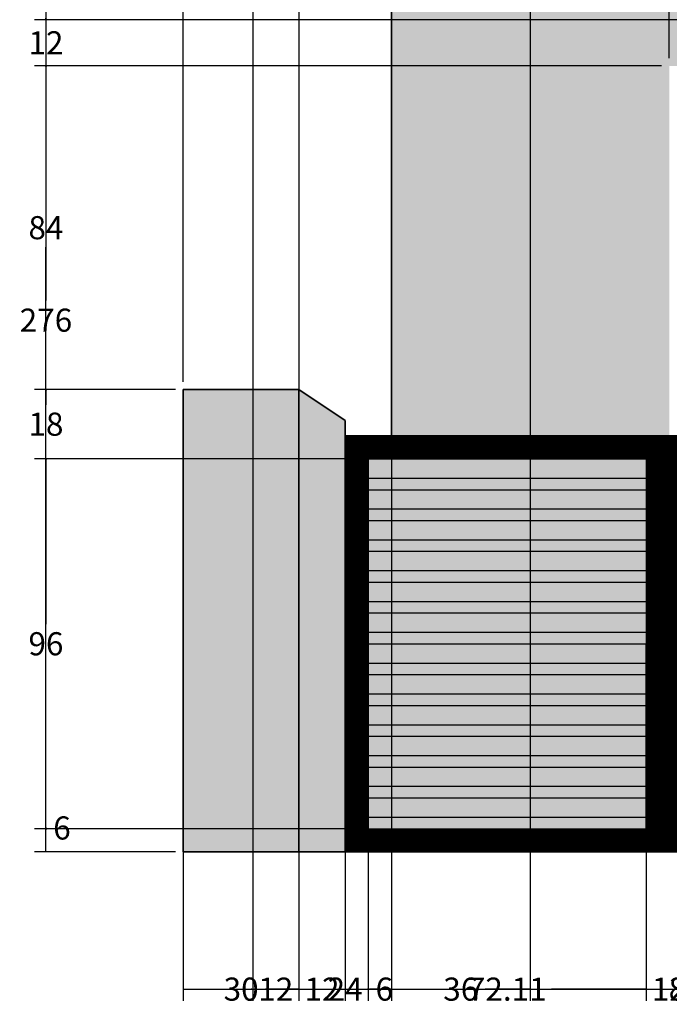
# Model space of a CAD drawing. Units: inches. Extents: x 860 to 1491, y 583 to 1370.
# Tile 1 of 8: x 866 to 1034, y 583 to 839. Entities that reach past the tile are written whole.
import ezdxf

# ---------------------------------------------------------------- set-up
doc = ezdxf.new("R2010")
doc.units = ezdxf.units.IN
doc.header["$MEASUREMENT"] = 0
doc.layers.get('0').update_dxf_attribs({"color": 250})
for name, color, linetype, lineweight in [('A-ANNO-DIMS', 2, 'Continuous', 18), ('A-ELEV', 7, 'Continuous', 35), ('A-ELEV-PATT', 9, 'Continuous', 13), ('A-SITE-GATE', 3, 'Continuous', 25), ('A-SITE-PATT', 8, 'Continuous', 13), ('A-SITE-WALL', 7, 'Continuous', 35)]:
    doc.layers.add(name, color=color, linetype=linetype, lineweight=lineweight)
doc.styles.get("Standard").update_dxf_attribs({"font": 'arial.ttf'})
doc.dimstyles.get("Standard").update_dxf_attribs({"dimtxt": 6, "dimasz": 0.18, "dimexe": 3, "dimexo": 2, "dimgap": 2, "dimtad": 0, "dimtih": 1, "dimtoh": 1, "dimdec": 0, "dimzin": 0, "dimdsep": 46, "dimlunit": 3, "dimtxsty": 'Standard', "dimblk2": 'CLOSEDBLANK', "dimsah": 1, "dimcen": 2, "dimadec": 0, "dimazin": 0, "dimtfac": 1, "dimtdec": 0, "dimtofl": 0, "dimtmove": 0, "dimatfit": 3, "dimfxl": 1, "dimtolj": 1, "dimtzin": 0, "dimarcsym": 0})

# ---------------------------------------------------------------- blocks, each defined once
blk = doc.blocks.new('_ClosedBlank')
at = {"color": 0, "linetype": 'ByBlock', "lineweight": -2}
for p, q in [((-1, 0.17), (0, 0)), ((-1, 0.17), (-1, -0.17)), ((0, 0), (-1, -0.17))]:
    blk.add_line(p, q, dxfattribs=at)
blk = doc.blocks.new('*D2')
at = {"layer": 'A-ANNO-DIMS', "color": 0, "lineweight": -2, "transparency": 16777216}
for p, q in [((1442.44, 1328.76), (1442.44, 584.11)), ((908.34, 740.76), (908.34, 584.11)), ((908.52, 587.11), (1163.85, 587.11)), ((1442.26, 587.11), (1186.93, 587.11))]:
    blk.add_line(p, q, dxfattribs=at)
at = {"layer": 'A-ANNO-DIMS', "color": 0, "transparency": 16777216}
blk.add_solid([(908.52, 587.14), (908.52, 587.08), (908.34, 587.11)], dxfattribs=at)
at = {"layer": 'Defpoints', "color": 0, "transparency": 16777216}
for p in [(1442.44, 1330.76), (908.34, 742.76), (1442.44, 587.11)]:
    blk.add_point(p, dxfattribs=at)
at = {"layer": 'A-ANNO-DIMS', "color": 0, "lineweight": -2, "transparency": 16777216, "xscale": 0.18, "yscale": 0.18, "zscale": 0.18}
blk.add_blockref('_ClosedBlank', (1442.44, 587.11), dxfattribs=at)
at = {"layer": 'A-ANNO-DIMS', "color": 0, "transparency": 16777216, "insert": (1175.39, 587.11), "char_height": 6, "attachment_point": 5}
blk.add_mtext('\\A1;534.1', dxfattribs=at)
blk = doc.blocks.new('*D4')
at = {"layer": 'A-ANNO-DIMS', "color": 0, "lineweight": -2, "transparency": 16777216}
for p, q in [((960.34, 898.76), (869.69, 898.76)), ((872.69, 898.58), (872.69, 765.82)), ((872.69, 622.94), (872.69, 755.69)), ((906.34, 622.76), (869.69, 622.76))]:
    blk.add_line(p, q, dxfattribs=at)
at = {"layer": 'A-ANNO-DIMS', "color": 0, "transparency": 16777216}
blk.add_solid([(872.66, 622.94), (872.72, 622.94), (872.69, 622.76)], dxfattribs=at)
at = {"layer": 'Defpoints', "color": 0, "transparency": 16777216}
for p in [(872.69, 898.76), (962.34, 898.76), (908.34, 622.76)]:
    blk.add_point(p, dxfattribs=at)
at = {"layer": 'A-ANNO-DIMS', "color": 0, "lineweight": -2, "transparency": 16777216, "xscale": 0.18, "yscale": 0.18, "zscale": 0.18, "rotation": 90}
blk.add_blockref('_ClosedBlank', (872.69, 898.76), dxfattribs=at)
at = {"layer": 'A-ANNO-DIMS', "color": 0, "transparency": 16777216, "insert": (872.69, 760.76), "char_height": 6, "attachment_point": 5}
blk.add_mtext('\\A1;276', dxfattribs=at)
blk = doc.blocks.new('*D6')
at = {"layer": 'A-ANNO-DIMS', "color": 0, "lineweight": -2, "transparency": 16777216}
for p, q in [((908.34, 740.76), (908.34, 584.11)), ((938.34, 740.76), (938.34, 584.11)), ((908.52, 587.11), (917.06, 587.11)), ((938.16, 587.11), (929.63, 587.11))]:
    blk.add_line(p, q, dxfattribs=at)
at = {"layer": 'A-ANNO-DIMS', "color": 0, "transparency": 16777216}
blk.add_solid([(908.52, 587.14), (908.52, 587.08), (908.34, 587.11)], dxfattribs=at)
at = {"layer": 'Defpoints', "color": 0, "transparency": 16777216}
for p in [(908.34, 742.76), (938.34, 742.76), (938.34, 587.11)]:
    blk.add_point(p, dxfattribs=at)
at = {"layer": 'A-ANNO-DIMS', "color": 0, "lineweight": -2, "transparency": 16777216, "xscale": 0.18, "yscale": 0.18, "zscale": 0.18}
blk.add_blockref('_ClosedBlank', (938.34, 587.11), dxfattribs=at)
at = {"layer": 'A-ANNO-DIMS', "color": 0, "transparency": 16777216, "insert": (923.34, 587.11), "char_height": 6, "attachment_point": 5}
blk.add_mtext('\\A1;30', dxfattribs=at)
blk = doc.blocks.new('*D7')
at = {"layer": 'A-ANNO-DIMS', "color": 0, "lineweight": -2, "transparency": 16777216}
for p, q in [((938.340309, 740.755507), (938.340309, 584.105507)), ((950.340309, 732.755507), (950.340309, 584.105507)), ((938.160309, 587.105507), (937.980309, 587.105507)), ((950.520309, 587.105507), (950.700309, 587.105507))]:
    blk.add_line(p, q, dxfattribs=at)
at = {"layer": 'A-ANNO-DIMS', "color": 0, "transparency": 16777216}
blk.add_solid([(938.160309, 587.135507), (938.160309, 587.075507), (938.340309, 587.105507)], dxfattribs=at)
at = {"layer": 'Defpoints', "color": 0, "transparency": 16777216}
for p in [(938.340309, 742.755507), (950.340309, 734.755507), (950.340309, 587.105507)]:
    blk.add_point(p, dxfattribs=at)
at = {"layer": 'A-ANNO-DIMS', "color": 0, "lineweight": -2, "transparency": 16777216, "xscale": 0.18, "yscale": 0.18, "zscale": 0.18, "rotation": 180}
blk.add_blockref('_ClosedBlank', (950.340309, 587.105507), dxfattribs=at)
at = {"layer": 'A-ANNO-DIMS', "color": 0, "transparency": 16777216, "insert": (944.340309, 587.105507), "char_height": 6, "attachment_point": 5}
blk.add_mtext('\\A1;12', dxfattribs=at)
blk = doc.blocks.new('*D8')
at = {"layer": 'A-ANNO-DIMS', "color": 0, "lineweight": -2, "transparency": 16777216}
for p, q in [((950.34, 732.76), (950.34, 584.11)), ((956.34, 722.76), (956.34, 584.11)), ((950.52, 587.11), (956.16, 587.11)), ((956.34, 587.11), (956.52, 587.11))]:
    blk.add_line(p, q, dxfattribs=at)
at = {"layer": 'A-ANNO-DIMS', "color": 0, "transparency": 16777216}
blk.add_solid([(950.52, 587.14), (950.52, 587.08), (950.34, 587.11)], dxfattribs=at)
at = {"layer": 'Defpoints', "color": 0, "transparency": 16777216}
for p in [(950.34, 734.76), (956.34, 724.76), (956.34, 587.11)]:
    blk.add_point(p, dxfattribs=at)
at = {"layer": 'A-ANNO-DIMS', "color": 0, "lineweight": -2, "transparency": 16777216, "xscale": 0.18, "yscale": 0.18, "zscale": 0.18}
blk.add_blockref('_ClosedBlank', (956.34, 587.11), dxfattribs=at)
at = {"layer": 'A-ANNO-DIMS', "color": 0, "transparency": 16777216, "insert": (960.5, 587.11), "char_height": 6, "attachment_point": 5}
blk.add_mtext('\\A1;6', dxfattribs=at)
blk = doc.blocks.new('*D9')
at = {"layer": 'A-ANNO-DIMS', "color": 0, "lineweight": -2, "transparency": 16777216}
for p, q in [((956.34, 722.76), (956.34, 584.11)), ((1028.45, 722.76), (1028.45, 584.11)), ((956.52, 587.11), (980.88, 587.11)), ((1028.27, 587.11), (1003.92, 587.11))]:
    blk.add_line(p, q, dxfattribs=at)
at = {"layer": 'A-ANNO-DIMS', "color": 0, "transparency": 16777216}
blk.add_solid([(956.52, 587.14), (956.52, 587.08), (956.34, 587.11)], dxfattribs=at)
at = {"layer": 'Defpoints', "color": 0, "transparency": 16777216}
for p in [(956.34, 724.76), (1028.45, 724.76), (1028.45, 587.11)]:
    blk.add_point(p, dxfattribs=at)
at = {"layer": 'A-ANNO-DIMS', "color": 0, "lineweight": -2, "transparency": 16777216, "xscale": 0.18, "yscale": 0.18, "zscale": 0.18}
blk.add_blockref('_ClosedBlank', (1028.45, 587.11), dxfattribs=at)
at = {"layer": 'A-ANNO-DIMS', "color": 0, "transparency": 16777216, "insert": (992.4, 587.11), "char_height": 6, "attachment_point": 5}
blk.add_mtext('\\A1;72.11', dxfattribs=at)
blk = doc.blocks.new('*D10')
at = {"layer": 'A-ANNO-DIMS', "color": 0, "lineweight": -2, "transparency": 16777216}
for p, q in [((1028.454444, 722.755507), (1028.454444, 584.105507)), ((1040.454446, 722.755507), (1040.454446, 584.105507)), ((1028.274444, 587.105507), (1028.094444, 587.105507)), ((1040.634446, 587.105507), (1040.814446, 587.105507))]:
    blk.add_line(p, q, dxfattribs=at)
at = {"layer": 'A-ANNO-DIMS', "color": 0, "transparency": 16777216}
blk.add_solid([(1028.274444, 587.135507), (1028.274444, 587.075507), (1028.454444, 587.105507)], dxfattribs=at)
at = {"layer": 'Defpoints', "color": 0, "transparency": 16777216}
for p in [(1028.454444, 724.755507), (1040.454446, 724.755507), (1040.454446, 587.105507)]:
    blk.add_point(p, dxfattribs=at)
at = {"layer": 'A-ANNO-DIMS', "color": 0, "lineweight": -2, "transparency": 16777216, "xscale": 0.18, "yscale": 0.18, "zscale": 0.18, "rotation": 180}
blk.add_blockref('_ClosedBlank', (1040.454446, 587.105507), dxfattribs=at)
at = {"layer": 'A-ANNO-DIMS', "color": 0, "transparency": 16777216, "insert": (1034.454445, 587.105507), "char_height": 6, "attachment_point": 5}
blk.add_mtext('\\A1;12', dxfattribs=at)
blk = doc.blocks.new('*D20')
at = {"layer": 'A-ANNO-DIMS', "color": 0, "lineweight": -2, "transparency": 16777216}
for p, q in [((908.34, 744.76), (908.34, 1369.41)), ((962.34, 732.76), (962.34, 1369.41)), ((908.52, 1366.41), (929.06, 1366.41)), ((962.16, 1366.41), (941.63, 1366.41))]:
    blk.add_line(p, q, dxfattribs=at)
at = {"layer": 'A-ANNO-DIMS', "color": 0, "transparency": 16777216}
blk.add_solid([(908.52, 1366.44), (908.52, 1366.38), (908.34, 1366.41)], dxfattribs=at)
at = {"layer": 'Defpoints', "color": 0, "transparency": 16777216}
for p in [(962.34, 1366.41), (908.34, 742.76), (962.34, 730.76)]:
    blk.add_point(p, dxfattribs=at)
at = {"layer": 'A-ANNO-DIMS', "color": 0, "lineweight": -2, "transparency": 16777216, "xscale": 0.18, "yscale": 0.18, "zscale": 0.18}
blk.add_blockref('_ClosedBlank', (962.34, 1366.41), dxfattribs=at)
at = {"layer": 'A-ANNO-DIMS', "color": 0, "transparency": 16777216, "insert": (935.34, 1366.41), "char_height": 6, "attachment_point": 5}
blk.add_mtext('\\A1;54', dxfattribs=at)
blk = doc.blocks.new('*D21')
at = {"layer": 'A-ANNO-DIMS', "color": 0, "lineweight": -2, "transparency": 16777216}
for p, q in [((962.34, 732.76), (962.34, 1369.41)), ((1034.46, 828.76), (1034.46, 1369.41)), ((962.52, 1366.41), (986.33, 1366.41)), ((1034.28, 1366.41), (1010.47, 1366.41))]:
    blk.add_line(p, q, dxfattribs=at)
at = {"layer": 'A-ANNO-DIMS', "color": 0, "transparency": 16777216}
blk.add_solid([(962.52, 1366.44), (962.52, 1366.38), (962.34, 1366.41)], dxfattribs=at)
at = {"layer": 'Defpoints', "color": 0, "transparency": 16777216}
for p in [(1034.46, 1366.41), (1034.46, 826.76), (962.34, 730.76)]:
    blk.add_point(p, dxfattribs=at)
at = {"layer": 'A-ANNO-DIMS', "color": 0, "lineweight": -2, "transparency": 16777216, "xscale": 0.18, "yscale": 0.18, "zscale": 0.18}
blk.add_blockref('_ClosedBlank', (1034.46, 1366.41), dxfattribs=at)
at = {"layer": 'A-ANNO-DIMS', "color": 0, "transparency": 16777216, "insert": (998.4, 1366.41), "char_height": 6, "attachment_point": 5}
blk.add_mtext('\\A1;72.12', dxfattribs=at)
blk = doc.blocks.new('*D22')
at = {"layer": 'A-ANNO-DIMS', "color": 0, "lineweight": -2, "transparency": 16777216}
for p, q in [((1034.46, 828.76), (1034.46, 1369.41)), ((1070.46, 828.76), (1070.46, 1369.41)), ((1034.64, 1366.41), (1046.17, 1366.41)), ((1070.28, 1366.41), (1058.75, 1366.41))]:
    blk.add_line(p, q, dxfattribs=at)
at = {"layer": 'A-ANNO-DIMS', "color": 0, "transparency": 16777216}
blk.add_solid([(1034.64, 1366.44), (1034.64, 1366.38), (1034.46, 1366.41)], dxfattribs=at)
at = {"layer": 'Defpoints', "color": 0, "transparency": 16777216}
for p in [(1070.46, 1366.41), (1034.46, 826.76), (1070.46, 826.76)]:
    blk.add_point(p, dxfattribs=at)
at = {"layer": 'A-ANNO-DIMS', "color": 0, "lineweight": -2, "transparency": 16777216, "xscale": 0.18, "yscale": 0.18, "zscale": 0.18}
blk.add_blockref('_ClosedBlank', (1070.46, 1366.41), dxfattribs=at)
at = {"layer": 'A-ANNO-DIMS', "color": 0, "transparency": 16777216, "insert": (1052.46, 1366.41), "char_height": 6, "attachment_point": 5}
blk.add_mtext('\\A1;36', dxfattribs=at)
blk = doc.blocks.new('*D31')
at = {"layer": 'A-ANNO-DIMS', "color": 0, "lineweight": -2, "transparency": 16777216}
for p, q in [((954.34, 628.76), (869.69, 628.76)), ((872.69, 628.76), (872.69, 628.94)), ((872.69, 628.94), (872.87, 628.94)), ((872.69, 622.94), (872.69, 628.58)), ((906.34, 622.76), (869.69, 622.76))]:
    blk.add_line(p, q, dxfattribs=at)
at = {"layer": 'A-ANNO-DIMS', "color": 0, "transparency": 16777216}
blk.add_solid([(872.66, 622.94), (872.72, 622.94), (872.69, 622.76)], dxfattribs=at)
at = {"layer": 'Defpoints', "color": 0, "transparency": 16777216}
for p in [(872.69, 628.76), (956.34, 628.76), (908.34, 622.76)]:
    blk.add_point(p, dxfattribs=at)
at = {"layer": 'A-ANNO-DIMS', "color": 0, "lineweight": -2, "transparency": 16777216, "xscale": 0.18, "yscale": 0.18, "zscale": 0.18, "rotation": 90}
blk.add_blockref('_ClosedBlank', (872.69, 628.76), dxfattribs=at)
at = {"layer": 'A-ANNO-DIMS', "color": 0, "transparency": 16777216, "insert": (876.85, 628.94), "char_height": 6, "attachment_point": 5}
blk.add_mtext('\\A1;6', dxfattribs=at)
blk = doc.blocks.new('*D32')
at = {"layer": 'A-ANNO-DIMS', "color": 0, "lineweight": -2, "transparency": 16777216}
for p, q in [((954.34, 724.76), (869.69, 724.76)), ((872.69, 724.58), (872.69, 681.82)), ((872.69, 628.94), (872.69, 671.69)), ((954.34, 628.76), (869.69, 628.76))]:
    blk.add_line(p, q, dxfattribs=at)
at = {"layer": 'A-ANNO-DIMS', "color": 0, "transparency": 16777216}
blk.add_solid([(872.66, 628.94), (872.72, 628.94), (872.69, 628.76)], dxfattribs=at)
at = {"layer": 'Defpoints', "color": 0, "transparency": 16777216}
for p in [(872.69, 724.76), (956.34, 724.76), (956.34, 628.76)]:
    blk.add_point(p, dxfattribs=at)
at = {"layer": 'A-ANNO-DIMS', "color": 0, "lineweight": -2, "transparency": 16777216, "xscale": 0.18, "yscale": 0.18, "zscale": 0.18, "rotation": 90}
blk.add_blockref('_ClosedBlank', (872.69, 724.76), dxfattribs=at)
at = {"layer": 'A-ANNO-DIMS', "color": 0, "transparency": 16777216, "insert": (872.69, 676.76), "char_height": 6, "attachment_point": 5}
blk.add_mtext('\\A1;96', dxfattribs=at)
blk = doc.blocks.new('*D33')
at = {"layer": 'A-ANNO-DIMS', "color": 0, "lineweight": -2, "transparency": 16777216}
for p, q in [((906.34, 742.76), (869.69, 742.76)), ((872.69, 742.58), (872.69, 738.82)), ((872.69, 724.94), (872.69, 728.69)), ((954.34, 724.76), (869.69, 724.76))]:
    blk.add_line(p, q, dxfattribs=at)
at = {"layer": 'A-ANNO-DIMS', "color": 0, "transparency": 16777216}
blk.add_solid([(872.66, 724.94), (872.72, 724.94), (872.69, 724.76)], dxfattribs=at)
at = {"layer": 'Defpoints', "color": 0, "transparency": 16777216}
for p in [(872.69, 742.76), (908.34, 742.76), (956.34, 724.76)]:
    blk.add_point(p, dxfattribs=at)
at = {"layer": 'A-ANNO-DIMS', "color": 0, "lineweight": -2, "transparency": 16777216, "xscale": 0.18, "yscale": 0.18, "zscale": 0.18, "rotation": 90}
blk.add_blockref('_ClosedBlank', (872.69, 742.76), dxfattribs=at)
at = {"layer": 'A-ANNO-DIMS', "color": 0, "transparency": 16777216, "insert": (872.69, 733.76), "char_height": 6, "attachment_point": 5}
blk.add_mtext('\\A1;18', dxfattribs=at)
blk = doc.blocks.new('*D34')
at = {"layer": 'A-ANNO-DIMS', "color": 0, "lineweight": -2, "transparency": 16777216}
for p, q in [((1032.46, 826.76), (869.69, 826.76)), ((872.69, 826.58), (872.69, 789.82)), ((872.69, 742.94), (872.69, 779.69)), ((906.34, 742.76), (869.69, 742.76))]:
    blk.add_line(p, q, dxfattribs=at)
at = {"layer": 'A-ANNO-DIMS', "color": 0, "transparency": 16777216}
blk.add_solid([(872.66, 742.94), (872.72, 742.94), (872.69, 742.76)], dxfattribs=at)
at = {"layer": 'Defpoints', "color": 0, "transparency": 16777216}
for p in [(872.69, 826.76), (1034.46, 826.76), (908.34, 742.76)]:
    blk.add_point(p, dxfattribs=at)
at = {"layer": 'A-ANNO-DIMS', "color": 0, "lineweight": -2, "transparency": 16777216, "xscale": 0.18, "yscale": 0.18, "zscale": 0.18, "rotation": 90}
blk.add_blockref('_ClosedBlank', (872.69, 826.76), dxfattribs=at)
at = {"layer": 'A-ANNO-DIMS', "color": 0, "transparency": 16777216, "insert": (872.69, 784.76), "char_height": 6, "attachment_point": 5}
blk.add_mtext('\\A1;84', dxfattribs=at)
blk = doc.blocks.new('*D35')
at = {"layer": 'A-ANNO-DIMS', "color": 0, "lineweight": -2, "transparency": 16777216}
for p, q in [((1116.440309, 838.755507), (869.690309, 838.755507)), ((872.690309, 838.935507), (872.690309, 839.115507)), ((1032.458453, 826.755507), (869.690309, 826.755507)), ((872.690309, 826.575507), (872.690309, 826.395507))]:
    blk.add_line(p, q, dxfattribs=at)
at = {"layer": 'A-ANNO-DIMS', "color": 0, "transparency": 16777216}
blk.add_solid([(872.660309, 826.575507), (872.720309, 826.575507), (872.690309, 826.755507)], dxfattribs=at)
at = {"layer": 'Defpoints', "color": 0, "transparency": 16777216}
for p in [(872.690309, 838.755507), (1118.440309, 838.755507), (1034.458453, 826.755507)]:
    blk.add_point(p, dxfattribs=at)
at = {"layer": 'A-ANNO-DIMS', "color": 0, "lineweight": -2, "transparency": 16777216, "xscale": 0.18, "yscale": 0.18, "zscale": 0.18, "rotation": 270}
blk.add_blockref('_ClosedBlank', (872.690309, 838.755507), dxfattribs=at)
at = {"layer": 'A-ANNO-DIMS', "color": 0, "transparency": 16777216, "insert": (872.690309, 832.755507), "char_height": 6, "attachment_point": 5}
blk.add_mtext('\\A1;12', dxfattribs=at)
blk = doc.blocks.new('*D62')
at = {"layer": 'A-ANNO-DIMS', "color": 0, "lineweight": -2, "transparency": 16777216}
for p, q in [((938.340309, 944.755507), (938.340309, 584.105507)), ((926.340309, 908.755507), (926.340309, 584.105507)), ((926.160309, 587.105507), (925.980309, 587.105507)), ((938.520309, 587.105507), (938.700309, 587.105507))]:
    blk.add_line(p, q, dxfattribs=at)
at = {"layer": 'A-ANNO-DIMS', "color": 0, "transparency": 16777216}
blk.add_solid([(926.160309, 587.135507), (926.160309, 587.075507), (926.340309, 587.105507)], dxfattribs=at)
at = {"layer": 'Defpoints', "color": 0, "transparency": 16777216}
for p in [(938.340309, 946.755507), (926.340309, 910.755507), (938.340309, 587.105507)]:
    blk.add_point(p, dxfattribs=at)
at = {"layer": 'A-ANNO-DIMS', "color": 0, "lineweight": -2, "transparency": 16777216, "xscale": 0.18, "yscale": 0.18, "zscale": 0.18, "rotation": 180}
blk.add_blockref('_ClosedBlank', (938.340309, 587.105507), dxfattribs=at)
at = {"layer": 'A-ANNO-DIMS', "color": 0, "transparency": 16777216, "insert": (932.340309, 587.105507), "char_height": 6, "attachment_point": 5}
blk.add_mtext('\\A1;12', dxfattribs=at)
blk = doc.blocks.new('*D63')
at = {"layer": 'A-ANNO-DIMS', "color": 0, "lineweight": -2, "transparency": 16777216}
for p, q in [((938.34, 944.76), (938.34, 584.11)), ((962.34, 881.35), (962.34, 584.11)), ((938.52, 587.11), (944, 587.11)), ((962.16, 587.11), (956.68, 587.11))]:
    blk.add_line(p, q, dxfattribs=at)
at = {"layer": 'A-ANNO-DIMS', "color": 0, "transparency": 16777216}
blk.add_solid([(938.52, 587.14), (938.52, 587.08), (938.34, 587.11)], dxfattribs=at)
at = {"layer": 'Defpoints', "color": 0, "transparency": 16777216}
for p in [(938.34, 946.76), (962.34, 883.35), (962.34, 587.11)]:
    blk.add_point(p, dxfattribs=at)
at = {"layer": 'A-ANNO-DIMS', "color": 0, "lineweight": -2, "transparency": 16777216, "xscale": 0.18, "yscale": 0.18, "zscale": 0.18}
blk.add_blockref('_ClosedBlank', (962.34, 587.11), dxfattribs=at)
at = {"layer": 'A-ANNO-DIMS', "color": 0, "transparency": 16777216, "insert": (950.34, 587.11), "char_height": 6, "attachment_point": 5}
blk.add_mtext('\\A1;24', dxfattribs=at)
blk = doc.blocks.new('*D64')
at = {"layer": 'A-ANNO-DIMS', "color": 0, "lineweight": -2, "transparency": 16777216}
for p, q in [((998.34, 956.76), (998.34, 584.11)), ((962.34, 881.35), (962.34, 584.11)), ((962.52, 587.11), (974.05, 587.11)), ((998.16, 587.11), (986.63, 587.11))]:
    blk.add_line(p, q, dxfattribs=at)
at = {"layer": 'A-ANNO-DIMS', "color": 0, "transparency": 16777216}
blk.add_solid([(962.52, 587.14), (962.52, 587.08), (962.34, 587.11)], dxfattribs=at)
at = {"layer": 'Defpoints', "color": 0, "transparency": 16777216}
for p in [(998.34, 958.76), (962.34, 883.35), (998.34, 587.11)]:
    blk.add_point(p, dxfattribs=at)
at = {"layer": 'A-ANNO-DIMS', "color": 0, "lineweight": -2, "transparency": 16777216, "xscale": 0.18, "yscale": 0.18, "zscale": 0.18}
blk.add_blockref('_ClosedBlank', (998.34, 587.11), dxfattribs=at)
at = {"layer": 'A-ANNO-DIMS', "color": 0, "transparency": 16777216, "insert": (980.34, 587.11), "char_height": 6, "attachment_point": 5}
blk.add_mtext('\\A1;36', dxfattribs=at)
blk = doc.blocks.new('*D65')
at = {"layer": 'A-ANNO-DIMS', "color": 0, "lineweight": -2, "transparency": 16777216}
for p, q in [((998.34, 956.76), (998.34, 584.11)), ((1079.34, 956.76), (1079.34, 584.11)), ((998.52, 587.11), (1033.12, 587.11)), ((1079.16, 587.11), (1044.56, 587.11))]:
    blk.add_line(p, q, dxfattribs=at)
at = {"layer": 'A-ANNO-DIMS', "color": 0, "transparency": 16777216}
blk.add_solid([(998.52, 587.14), (998.52, 587.08), (998.34, 587.11)], dxfattribs=at)
at = {"layer": 'Defpoints', "color": 0, "transparency": 16777216}
for p in [(998.34, 958.76), (1079.34, 958.76), (1079.34, 587.11)]:
    blk.add_point(p, dxfattribs=at)
at = {"layer": 'A-ANNO-DIMS', "color": 0, "lineweight": -2, "transparency": 16777216, "xscale": 0.18, "yscale": 0.18, "zscale": 0.18}
blk.add_blockref('_ClosedBlank', (1079.34, 587.11), dxfattribs=at)
at = {"layer": 'A-ANNO-DIMS', "color": 0, "transparency": 16777216, "insert": (1038.84, 587.11), "char_height": 6, "attachment_point": 5}
blk.add_mtext('\\A1;81', dxfattribs=at)

msp = doc.modelspace()

# ---------------------------------------------------------------- hatches: boundary and pattern name
at = {"layer": 'A-ELEV-PATT'}
h = msp.add_hatch(color=256, dxfattribs=at)
h.dxf.hatch_style = 1
h.paths.add_polyline_path([(1442.4403, 1330.7555), (1370.4403, 1330.7555), (1370.4403, 622.7555), (1442.4403, 622.7555)])
h.paths.add_polyline_path([(1358.4403, 1306.7555), (1190.4403, 1306.7555), (1190.4403, 1288.7555), (1358.4403, 1288.7555)])
h.paths.add_polyline_path([(1190.4403, 1234.7555), (962.3403, 1234.7555), (962.3403, 1198.7555), (1202.4403, 1198.7555), (1202.4403, 1216.7555), (1190.4403, 1216.7555)])
h.paths.add_polyline_path([(1202.4403, 1117.6207), (962.3403, 1117.6207), (962.3403, 982.7555), (986.3403, 982.7555), (986.3403, 1090.7555), (1178.3403, 1090.7555), (1178.3403, 982.7555), (1202.4403, 982.7555)])
h.paths.add_polyline_path([(1319.4403, 1184.7555), (1202.4403, 1184.7555), (1202.4403, 982.7555), (1211.4403, 982.7555), (1211.4403, 946.7555), (1220.4403, 946.7555), (1220.4403, 934.7555), (1319.4403, 934.7555)])
h.paths.add_polyline_path([(1271.4403, 1160.7555), (1307.4403, 1160.7555), (1307.4403, 944.7555), (1271.4403, 944.7555)], flags=16)
h.paths.add_polyline_path([(1275.4403, 1156.7555), (1303.4403, 1156.7555), (1303.4403, 948.7555), (1275.4403, 948.7555)], flags=0)
h.paths.add_polyline_path([(1202.4403, 898.7555), (962.3403, 898.7555), (962.3403, 730.7555), (1034.4585, 730.7555), (1034.4585, 826.7555), (1070.4585, 826.7555), (1070.4585, 730.7555), (1118.4403, 730.7555), (1118.4403, 838.7555), (1178.4403, 838.7555), (1178.4403, 730.7555), (1202.4403, 730.7555)])
h.paths.add_polyline_path([(1220.4403, 946.7555), (1211.4403, 946.7555), (938.3403, 946.7555), (926.3403, 946.7555), (926.3403, 910.7555), (962.3403, 910.7555), (1220.4403, 910.7555)])
h.paths.add_polyline_path([(950.3403, 730.7555), (950.3403, 734.7555), (938.3403, 742.7555), (938.3403, 730.7555), (938.3403, 622.7555), (950.3403, 622.7555)])
h = msp.add_hatch(color=256, dxfattribs=at)
h.dxf.hatch_style = 1
h.paths.add_polyline_path([(1370.4403, 730.7555), (1232.4403, 730.7555), (1232.4403, 622.7555), (1370.4403, 622.7555)])
h.paths.add_polyline_path([(1232.4403, 730.7555), (1232.4403, 742.7555), (1202.4403, 742.7555), (1202.4403, 622.7555), (1232.4403, 622.7555)])
h.paths.add_polyline_path([(1148.4403, 730.7555), (1148.4403, 742.7555), (1118.4403, 742.7555), (1118.4403, 718.7555), (1118.4403, 622.7555), (1148.4403, 622.7555)])
h.paths.add_polyline_path([(938.3403, 730.7555), (938.3403, 742.7555), (908.3403, 742.7555), (908.3403, 736.7555), (908.3403, 622.7555), (938.3403, 622.7555)])
h = msp.add_hatch(color=256, dxfattribs=at)
h.paths.add_polyline_path([(1040.4544, 724.7555), (1040.4511, 719.7555), (1112.4403, 719.7555), (1112.4403, 724.7555)])
h.paths.add_polyline_path([(1028.4511, 719.7555), (1028.4544, 724.7555), (956.3403, 724.7555), (956.3403, 719.7555)])
h.paths.add_polyline_path([(1028.4458, 711.7555), (1028.4491, 716.7555), (956.3403, 716.7555), (956.3403, 711.7555)])
h.paths.add_polyline_path([(1040.4491, 716.7555), (1040.4458, 711.7555), (1112.4403, 711.7555), (1112.4403, 716.7555)])
h.paths.add_polyline_path([(1040.4438, 708.7555), (1040.4404, 703.7555), (1112.4403, 703.7555), (1112.4403, 708.7555)])
h.paths.add_polyline_path([(1028.4351, 695.7555), (1028.4384, 700.7555), (956.3403, 700.7555), (956.3403, 695.7555)])
h.paths.add_polyline_path([(1040.4331, 692.7555), (1040.4297, 687.7555), (1112.4403, 687.7555), (1112.4403, 692.7555)])
h.paths.add_polyline_path([(1040.4224, 676.7555), (1040.419, 671.7555), (1112.4403, 671.7555), (1112.4403, 676.7555)])
h.paths.add_polyline_path([(1040.417, 668.7555), (1040.4137, 663.7555), (1112.4403, 663.7555), (1112.4403, 668.7555)])
h.paths.add_polyline_path([(1040.4063, 652.7555), (1040.403, 647.7555), (1112.4403, 647.7555), (1112.4403, 652.7555)])
h.paths.add_polyline_path([(1040.3957, 636.7555), (1040.3923, 631.7555), (1112.4403, 631.7555), (1112.4403, 636.7555)])
h = msp.add_hatch(color=256, dxfattribs=at)
h.paths.add_polyline_path([(1028.4511, 719.7555), (956.3403, 719.7555), (956.3403, 716.7555), (1028.4491, 716.7555)])
h.paths.add_polyline_path([(1028.4458, 711.7555), (956.3403, 711.7555), (956.3403, 708.7555), (1028.4438, 708.7555)])
h.paths.add_polyline_path([(1028.4404, 703.7555), (956.3403, 703.7555), (956.3403, 700.7555), (1028.4384, 700.7555)])
h.paths.add_polyline_path([(1028.4351, 695.7555), (956.3403, 695.7555), (956.3403, 692.7555), (1028.4331, 692.7555)])
h.paths.add_polyline_path([(1028.4297, 687.7555), (956.3403, 687.7555), (956.3403, 684.7555), (1028.4277, 684.7555)])
h.paths.add_polyline_path([(1028.4244, 679.7555), (956.3403, 679.7555), (956.3403, 676.7555), (1028.4224, 676.7555)])
h.paths.add_polyline_path([(1028.419, 671.7555), (956.3403, 671.7555), (956.3403, 668.7555), (1028.417, 668.7555)])
h.paths.add_polyline_path([(1028.4137, 663.7555), (956.3403, 663.7555), (956.3403, 660.7555), (1028.4117, 660.7555)])
h.paths.add_polyline_path([(1028.4083, 655.7555), (956.3403, 655.7555), (956.3403, 652.7555), (1028.4063, 652.7555)])
h.paths.add_polyline_path([(1028.403, 647.7555), (956.3403, 647.7555), (956.3403, 644.7555), (1028.401, 644.7555)])
h.paths.add_polyline_path([(1028.3977, 639.7555), (956.3403, 639.7555), (956.3403, 636.7555), (1028.3957, 636.7555)])
h.paths.add_polyline_path([(1028.3923, 631.7555), (956.3403, 631.7555), (956.3403, 628.7555), (1028.3903, 628.7074)])
h.paths.add_polyline_path([(1112.4403, 719.7555), (1040.4511, 719.7555), (1040.4491, 716.7555), (1112.4403, 716.7555)])
h.paths.add_polyline_path([(1112.4403, 711.7555), (1040.4458, 711.7555), (1040.4438, 708.7555), (1112.4403, 708.7555)])
h.paths.add_polyline_path([(1112.4403, 703.7555), (1040.4404, 703.7555), (1040.4384, 700.7555), (1112.4403, 700.7555)])
h.paths.add_polyline_path([(1112.4403, 695.7555), (1040.4351, 695.7555), (1040.4331, 692.7555), (1112.4403, 692.7555)])
h.paths.add_polyline_path([(1112.4403, 687.7555), (1040.4297, 687.7555), (1040.4277, 684.7555), (1112.4403, 684.7555)])
h.paths.add_polyline_path([(1112.4403, 679.7555), (1040.4244, 679.7555), (1040.4224, 676.7555), (1112.4403, 676.7555)])
h.paths.add_polyline_path([(1112.4403, 671.7555), (1040.419, 671.7555), (1040.417, 668.7555), (1112.4403, 668.7555)])
h.paths.add_polyline_path([(1112.4403, 663.7555), (1040.4137, 663.7555), (1040.4117, 660.7555), (1112.4403, 660.7555)])
h.paths.add_polyline_path([(1112.4403, 655.7555), (1040.4083, 655.7555), (1040.4063, 652.7555), (1112.4403, 652.7555)])
h.paths.add_polyline_path([(1112.4403, 647.7555), (1040.403, 647.7555), (1040.401, 644.7555), (1112.4403, 644.7555)])
h.paths.add_polyline_path([(1112.4403, 639.7555), (1040.3977, 639.7555), (1040.3957, 636.7555), (1112.4403, 636.7555)])
h.paths.add_polyline_path([(1112.4403, 631.7555), (1040.3923, 631.7555), (1040.3903, 628.7555), (1112.4403, 628.7555)])
h.paths.add_polyline_path([(1196.4403, 719.7555), (1154.4403, 719.7555), (1154.4403, 716.7555), (1196.4403, 716.7555)])
h.paths.add_polyline_path([(1196.4403, 711.7555), (1154.4403, 711.7555), (1154.4403, 708.7555), (1196.4403, 708.7555)])
h.paths.add_polyline_path([(1196.4403, 703.7555), (1154.4403, 703.7555), (1154.4403, 700.7555), (1196.4403, 700.7555)])
h.paths.add_polyline_path([(1196.4403, 695.7555), (1154.4403, 695.7555), (1154.4403, 692.7555), (1196.4403, 692.7555)])
h.paths.add_polyline_path([(1196.4403, 687.7555), (1154.4403, 687.7555), (1154.4403, 684.7555), (1196.4403, 684.7555)])
h.paths.add_polyline_path([(1196.4403, 679.7555), (1154.4403, 679.7555), (1154.4403, 676.7555), (1196.4403, 676.7555)])
h.paths.add_polyline_path([(1196.4403, 671.7555), (1154.4403, 671.7555), (1154.4403, 668.7555), (1196.4403, 668.7555)])
h.paths.add_polyline_path([(1196.4403, 663.7555), (1154.4403, 663.7555), (1154.4403, 660.7555), (1196.4403, 660.7555)])
h.paths.add_polyline_path([(1196.4403, 655.7555), (1154.4403, 655.7555), (1154.4403, 652.7555), (1196.4403, 652.7555)])
h.paths.add_polyline_path([(1196.4403, 647.7555), (1154.4403, 647.7555), (1154.4403, 644.7555), (1196.4403, 644.7555)])
h.paths.add_polyline_path([(1196.4403, 639.7555), (1154.4403, 639.7555), (1154.4403, 636.7555), (1196.4403, 636.7555)])
h.paths.add_polyline_path([(1196.4403, 631.7555), (1154.4403, 631.7555), (1154.4403, 628.7555), (1196.4403, 628.7555)])
h = msp.add_hatch(color=256, dxfattribs=at)
h.paths.add_polyline_path([(1028.4438, 708.7555), (956.3403, 708.7555), (956.3403, 703.7555), (1028.4404, 703.7555)])
h.paths.add_polyline_path([(1028.4331, 692.7555), (956.3403, 692.7555), (956.3403, 687.7555), (1028.4297, 687.7555)])
h.paths.add_polyline_path([(1028.4277, 684.7555), (956.3403, 684.7555), (956.3403, 679.7555), (1028.4244, 679.7555)])
h.paths.add_polyline_path([(1028.4224, 676.7555), (956.3403, 676.7555), (956.3403, 671.7555), (1028.419, 671.7555)])
h.paths.add_polyline_path([(1028.417, 668.7555), (956.3403, 668.7555), (956.3403, 663.7555), (1028.4137, 663.7555)])
h.paths.add_polyline_path([(1028.4117, 660.7555), (956.3403, 660.7555), (956.3403, 655.7555), (1028.4083, 655.7555)])
h.paths.add_polyline_path([(1028.4063, 652.7555), (956.3403, 652.7555), (956.3403, 647.7555), (1028.403, 647.7555)])
h.paths.add_polyline_path([(1028.401, 644.7555), (956.3403, 644.7555), (956.3403, 639.7555), (1028.3977, 639.7555)])
h.paths.add_polyline_path([(1028.3957, 636.7555), (956.3403, 636.7555), (956.3403, 631.7555), (1028.3923, 631.7555)])
h.paths.add_polyline_path([(1112.4403, 644.7555), (1040.401, 644.7555), (1040.3977, 639.7555), (1112.4403, 639.7555)])
h.paths.add_polyline_path([(1112.4403, 660.7555), (1040.4117, 660.7555), (1040.4083, 655.7555), (1112.4403, 655.7555)])
h.paths.add_polyline_path([(1112.4403, 684.7555), (1040.4277, 684.7555), (1040.4244, 679.7555), (1112.4403, 679.7555)])
h.paths.add_polyline_path([(1112.4403, 700.7555), (1040.4384, 700.7555), (1040.4351, 695.7555), (1112.4403, 695.7555)])
at = {"layer": 'A-SITE-PATT'}
h = msp.add_hatch(dxfattribs=at)
h.set_pattern_fill('GRAVEL', color=256, scale=30, style=0)
h.set_pattern_definition([(228.01279, (21.6, 30), (-240, -270), [4.0361, -399.57264]), (184.96974, (18.9, 27), (360, 30), [6.92604, -685.67774]), (132.51045, (12, 26.4), (300, -330), [4.88364, -483.481]), (267.27369, (0.3, 18.9), (30, 600), [6.30714, -624.40674]), (292.83365, (0, 12.6), (-150, 360), [6.18465, -612.2812]), (357.27369, (2.4, 6.9), (-600, 30), [6.30714, -624.40674]), (37.69424, (8.7, 6.6), (-390, -300), [8.34087, -825.74546]), (72.25533, (15.3, 11.7), (210, 660), [7.87464, -779.58964]), (121.42957, (17.7, 19.2), (-240, 390), [6.3285, -626.5222]), (175.23636, (14.4, 24.6), (330, -30), [7.22496, -354.0229]), (222.39744, (7.2, 25.2), (-360, -330), [9.34344, -925.00125]), (138.81407, (30, 18.6), (-210, 180), [3.18903, -315.71534]), (171.46923, (27.6, 20.7), (390, -60), [6.0671, -600.64534]), (225, (21.6, 21.6), (-3e-15, -30), [4.24263, -38.1838]), (203.1986, (19.5, 25.2), (150, 60), [2.28474, -226.18845]), (291.8014, (17.4, 24.3), (-30, 90), [3.2311, -158.32385]), (30.96376, (18.6, 21.3), (90, 60), [5.24787, -169.6807]), (161.56505, (23.1, 24), (60, -30), [3.79473, -91.0736]), (16.38954, (0, 24.3), (300, 90), [5.316, -526.28535]), (70.34618, (5.1, 25.8), (-120, -330), [4.45983, -441.52223]), (293.1986, (23.1, 30), (-60, 150), [4.56945, -223.90374]), (343.61046, (24.9, 25.8), (-300, 90), [5.316, -526.28535]), (339.44395, (0, 5.7), (-150, 60), [5.1264, -251.1937]), (294.77514, (4.8, 3.9), (-150, 330), [4.29534, -425.2393]), (66.8014, (23.4, 0), (60, 150), [4.56945, -223.90374]), (17.35402, (25.2, 4.2), (-390, -120), [5.02893, -497.8627]), (69.44395, (8.7, 0), (-60, -150), [2.5632, -253.7569]), (101.30993, (21.6, 0), (-30, 120), [1.5297, -151.4409]), (165.96376, (21.3, 1.5), (90, -30), [6.18465, -117.5085]), (186.00901, (15.3, 3), (300, 30), [5.7315, -567.4177]), (303.69007, (18.6, 18.6), (-30, 60), [4.32666, -103.8399]), (353.15723, (21, 15), (510, -60), [7.55382, -747.82688]), (60.9454, (28.5, 14.1), (-120, -210), [3.0887, -305.7802]), (90, (30, 16.8), (-30, 30), [1.8, -28.2]), (120.25644, (14.7, 3.9), (120, -210), [4.1677, -412.6056]), (48.01279, (12.6, 7.5), (240, 270), [8.07216, -395.53656]), (0, (18, 13.5), (30, 30), [7.8, -22.2]), (325.30485, (25.8, 13.5), (300, -210), [4.7434, -469.59823]), (254.0546, (29.7, 10.8), (-30, -120), [4.36806, -214.03524]), (207.64598, (28.5, 6.6), (-570, -300), [7.11195, -704.08423]), (175.42608, (22.2, 3.3), (-390, 30), [7.52397, -744.8722])])
h.paths.add_polyline_path([(1370.4403, 730.7555), (1232.4403, 730.7555), (1232.4403, 622.7555), (1370.4403, 622.7555)])
h.paths.add_polyline_path([(1232.4403, 730.7555), (1232.4403, 742.7555), (1202.4403, 742.7555), (1202.4403, 622.7555), (1232.4403, 622.7555)])
h.paths.add_polyline_path([(1148.4403, 730.7555), (1148.4403, 742.7555), (1118.4403, 742.7555), (1118.4403, 718.7555), (1118.4403, 622.7555), (1148.4403, 622.7555)])
h.paths.add_polyline_path([(938.3403, 730.7555), (938.3403, 742.7555), (908.3403, 742.7555), (908.3403, 736.7555), (908.3403, 622.7555), (938.3403, 622.7555)])
h = msp.add_hatch(dxfattribs=at)
h.set_pattern_fill('ANSI31', color=256, style=0)
h.paths.add_polyline_path([(1118.4403, 730.7555), (962.3403, 730.7555), (950.3403, 730.7555), (950.3403, 622.7555), (1118.4403, 622.7555)])
h.paths.add_polyline_path([(1028.4544, 724.7555), (1028.3903, 628.7074), (956.3403, 628.7555), (956.3403, 724.7555)], flags=16)
h.paths.add_polyline_path([(1040.4544, 724.7555), (1112.4403, 724.7555), (1112.4403, 628.7555), (1040.3903, 628.7555)], flags=16)
h.paths.add_polyline_path([(1202.4403, 730.7555), (1148.4403, 730.7555), (1148.4403, 622.7555), (1202.4403, 622.7555)])
h.paths.add_polyline_path([(1154.4403, 724.7555), (1196.4403, 724.7555), (1196.4403, 628.7555), (1154.4403, 628.7555)], flags=16)

# ---------------------------------------------------------------- linework, layer by layer
at = {"layer": 'A-ELEV'}
for p, q in [((962.3403, 730.7555), (962.3403, 898.7555)), ((938.3403, 742.7555), (908.3403, 742.7555)), ((908.3403, 742.7555), (908.3403, 736.7555)), ((938.3403, 730.7555), (938.3403, 742.7555)), ((950.3403, 734.7555), (938.3403, 742.7555)), ((908.3403, 622.7555), (908.3403, 736.7555)), ((950.3403, 730.7555), (950.3403, 734.7555))]:
    msp.add_line(p, q, dxfattribs=at)
at = {"layer": 'A-SITE-GATE'}
for p, q in [((956.3403, 724.7555), (956.3403, 628.7555)), ((956.3403, 724.7555), (1028.4544, 724.7555)), ((1028.4544, 724.7555), (1028.3903, 628.7595)), ((956.3403, 719.7555), (1028.4511, 719.7555)), ((956.3403, 716.7555), (1028.4491, 716.7555)), ((956.3403, 711.7555), (1028.4458, 711.7555)), ((956.3403, 708.7555), (1028.4438, 708.7555)), ((956.3403, 703.7555), (1028.4404, 703.7555)), ((956.3403, 700.7555), (1028.4384, 700.7555)), ((956.3403, 695.7555), (1028.4351, 695.7555)), ((956.3403, 692.7555), (1028.4331, 692.7555)), ((956.3403, 687.7555), (1028.4297, 687.7555)), ((956.3403, 684.7555), (1028.4277, 684.7555)), ((956.3403, 679.7555), (1028.4244, 679.7555)), ((956.3403, 676.7555), (1028.4224, 676.7555)), ((956.3403, 671.7555), (1028.419, 671.7555)), ((956.3403, 668.7555), (1028.417, 668.7555)), ((956.3403, 663.7555), (1028.4137, 663.7555)), ((956.3403, 660.7555), (1028.4117, 660.7555)), ((956.3403, 655.7555), (1028.4083, 655.7555)), ((956.3403, 652.7555), (1028.4063, 652.7555)), ((956.3403, 647.7555), (1028.403, 647.7555)), ((956.3403, 644.7555), (1028.401, 644.7555)), ((956.3403, 639.7555), (1028.3977, 639.7555)), ((956.3403, 636.7555), (1028.3957, 636.7555)), ((956.3403, 631.7555), (1028.3923, 631.7555)), ((956.3403, 628.7555), (1028.3903, 628.7074))]:
    msp.add_line(p, q, dxfattribs=at)
at = {"layer": 'A-SITE-WALL'}
for p, q in [((938.3403, 622.7555), (938.3403, 730.7555)), ((962.3403, 730.7555), (950.3403, 730.7555)), ((950.3403, 730.7555), (950.3403, 622.7555)), ((962.3403, 730.7555), (1118.4403, 730.7555)), ((1028.4585, 730.7595), (1028.4585, 730.7555)), ((908.3403, 622.7555), (1442.4403, 622.7555))]:
    msp.add_line(p, q, dxfattribs=at)

# ---------------------------------------------------------------- dimensions: what is measured, and where the dimension line sits
at = {"layer": 'A-ANNO-DIMS'}
for base, p1, p2, override, picture, middle in [((962.3403, 1366.4055), (908.3403, 742.7555), (962.3403, 730.7555), {"dimdec": 0, "dimlfac": 1, "dimrnd": 0, "dimzin": 0, "dimdsep": 46, "dimlunit": 2}, '*D20', (935.3403, 1366.4055)), ((1034.4585, 1366.4055), (962.3403, 730.7555), (1034.4585, 826.7555), {"dimdec": 2, "dimlfac": 1, "dimrnd": 0, "dimzin": 0, "dimdsep": 46, "dimlunit": 2}, '*D21', (998.3994, 1366.4055)), ((1070.4585, 1366.4055), (1034.4585, 826.7555), (1070.4585, 826.7555), {"dimdec": 0, "dimlfac": 1, "dimrnd": 0, "dimzin": 0, "dimdsep": 46, "dimlunit": 2}, '*D22', (1052.4585, 1366.4055)), ((1442.4403, 587.1055), (908.3403, 742.7555), (1442.4403, 1330.7555), {"dimdec": 1, "dimlfac": 1, "dimrnd": 0, "dimzin": 0, "dimdsep": 46, "dimlunit": 2}, '*D2', (1175.3903, 587.1055)), ((998.3403, 587.1055), (962.3403, 883.3536), (998.3403, 958.7555), {"dimdec": 0, "dimlfac": 1, "dimrnd": 0, "dimzin": 0, "dimdsep": 46, "dimlunit": 2}, '*D64', (980.3403, 587.1055)), ((1079.3403, 587.1055), (998.3403, 958.7555), (1079.3403, 958.7555), {"dimdec": 0, "dimlfac": 1, "dimrnd": 0, "dimzin": 0, "dimdsep": 46, "dimlunit": 2}, '*D65', (1038.8403, 587.1055)), ((938.3403, 587.1055), (926.3403, 910.7555), (938.3403, 946.7555), {"dimdec": 0, "dimlfac": 1, "dimrnd": 0, "dimzin": 0, "dimdsep": 46, "dimlunit": 2}, '*D62', (932.3403, 587.1055)), ((962.3403, 587.1055), (938.3403, 946.7555), (962.3403, 883.3536), {"dimdec": 0, "dimlfac": 1, "dimrnd": 0, "dimzin": 0, "dimdsep": 46, "dimlunit": 2}, '*D63', (950.3403, 587.1055)), ((938.3403, 587.1055), (908.3403, 742.7555), (938.3403, 742.7555), {"dimdec": 0, "dimlfac": 1, "dimrnd": 0, "dimzin": 0, "dimdsep": 46, "dimlunit": 2}, '*D6', (923.3403, 587.1055)), ((950.3403, 587.1055), (938.3403, 742.7555), (950.3403, 734.7555), {"dimdec": 0, "dimlfac": 1, "dimrnd": 0, "dimzin": 0, "dimdsep": 46, "dimlunit": 2}, '*D7', (944.3403, 587.1055)), ((956.3403, 587.1055), (950.3403, 734.7555), (956.3403, 724.7555), {"dimdec": 0, "dimlfac": 1, "dimrnd": 0, "dimzin": 0, "dimdsep": 46, "dimlunit": 2}, '*D8', (960.5012, 587.1055)), ((1028.4544, 587.1055), (956.3403, 724.7555), (1028.4544, 724.7555), {"dimdec": 2, "dimlfac": 1, "dimrnd": 0, "dimzin": 0, "dimdsep": 46, "dimlunit": 2}, '*D9', (992.3974, 587.1055)), ((1040.4544, 587.1055), (1028.4544, 724.7555), (1040.4544, 724.7555), {"dimdec": 0, "dimlfac": 1, "dimrnd": 0, "dimzin": 0, "dimdsep": 46, "dimlunit": 2}, '*D10', (1034.4544, 587.1055))]:
    dim = msp.add_linear_dim(base=base, p1=p1, p2=p2, dimstyle='Standard', override=override, dxfattribs=at)
    dim.commit()
    dim.dimension.update_dxf_attribs({"geometry": picture, "text_midpoint": middle})
for base, p1, p2, picture, middle in [((872.6903, 898.7555), (908.3403, 622.7555), (962.3403, 898.7555), '*D4', (872.6903, 760.7555)), ((872.6903, 838.7555), (1034.4585, 826.7555), (1118.4403, 838.7555), '*D35', (872.6903, 832.7555)), ((872.6903, 826.7555), (908.3403, 742.7555), (1034.4585, 826.7555), '*D34', (872.6903, 784.7555)), ((872.6903, 742.7555), (956.3403, 724.7555), (908.3403, 742.7555), '*D33', (872.6903, 733.7555)), ((872.6903, 724.7555), (956.3403, 628.7555), (956.3403, 724.7555), '*D32', (872.6903, 676.7555)), ((872.6903, 628.7555), (908.3403, 622.7555), (956.3403, 628.7555), '*D31', (876.8512, 628.9355))]:
    dim = msp.add_linear_dim(base=base, p1=p1, p2=p2, angle=90, dimstyle='Standard', override={"dimdec": 0, "dimlfac": 1, "dimrnd": 0, "dimzin": 0, "dimdsep": 46, "dimlunit": 2}, dxfattribs=at)
    dim.commit()
    dim.dimension.update_dxf_attribs({"geometry": picture, "text_midpoint": middle})

doc.saveas('drawing.dxf')
